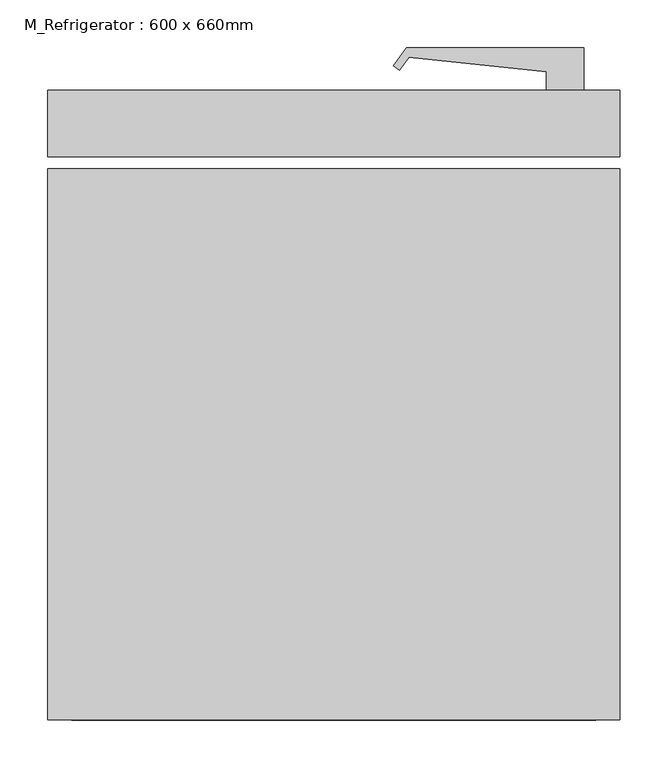
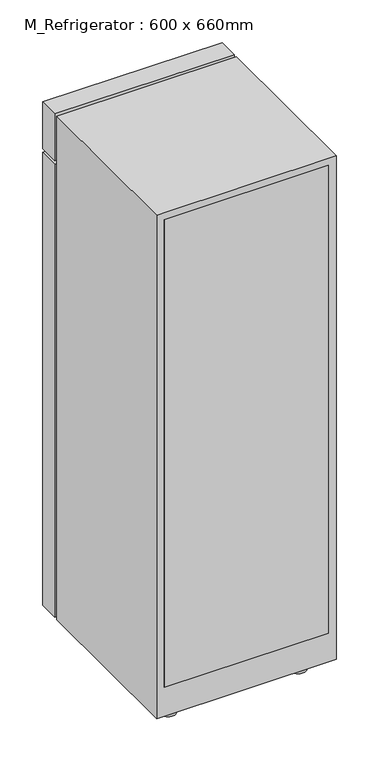
"""IFC4 building model written with IfcOpenShell, lengths in millimetres: proxy geometry, M_Refrigerator : 600 x 660mm."""

from ifc_helpers import new_model, si_unit, point, frame, frame_2d, origin, origin_with_axes, place, context, project, spatial, polyline, circle_curve, trimmed, segment, composite_curve, outline, extrude, source, transform, mapped, element, save


def m_refrigerator_600_x_660mm_0a899b9c(model_context):
    return source(origin(), model_context, "Body", "SweptSolid", [
        extrude(outline(polyline([(208.0988574, 408.1036861), (208.0988574, 363.7849098), (168.9242419, 363.7849098), (168.9242419, 383.0358618), (25.1756383, 398.2543926), (15.2273026, 384.7471068), (8.7240737, 389.5368406), (22.3988574, 408.1036861), (208.0988574, 408.1036861)])), frame((0.0, 0.0, 1071.927792), z_axis=(0.0, 0.0, 1.0), x_axis=(1.0, 0.0, 0.0)), (0.0, 0.0, 1.0), 31.75),
        extrude(outline(composite_curve([segment(trimmed(circle_curve(frame_2d((-271.2511426, -220.0150902)), 25.4), [point((-296.6511426, -220.0150902))], [point((-245.8511426, -220.0150902))], False, "CARTESIAN"), True, "CONTINUOUS"), segment(trimmed(circle_curve(frame_2d((-271.2511426, -220.0150902)), 25.4), [point((-245.8511426, -220.0150902))], [point((-296.6511426, -220.0150902))], False, "CARTESIAN"), True, "CONTINUOUS")], self_intersect=False)), origin_with_axes(), (0.0, 0.0, 1.0), 50.8),
        extrude(outline(composite_curve([segment(trimmed(circle_curve(frame_2d((163.6488574, -220.0150902)), 25.4), [point((138.2488574, -220.0150902))], [point((189.0488574, -220.0150902))], False, "CARTESIAN"), True, "CONTINUOUS"), segment(trimmed(circle_curve(frame_2d((163.6488574, -220.0150902)), 25.4), [point((189.0488574, -220.0150902))], [point((138.2488574, -220.0150902))], False, "CARTESIAN"), True, "CONTINUOUS")], self_intersect=False)), origin_with_axes(), (0.0, 0.0, 1.0), 50.8),
        extrude(outline(composite_curve([segment(trimmed(circle_curve(frame_2d((-271.2511426, 236.7849098)), 25.4), [point((-296.6511426, 236.7849098))], [point((-245.8511426, 236.7849098))], False, "CARTESIAN"), True, "CONTINUOUS"), segment(trimmed(circle_curve(frame_2d((-271.2511426, 236.7849098)), 25.4), [point((-245.8511426, 236.7849098))], [point((-296.6511426, 236.7849098))], False, "CARTESIAN"), True, "CONTINUOUS")], self_intersect=False)), origin_with_axes(), (0.0, 0.0, 1.0), 50.8),
        extrude(outline(composite_curve([segment(trimmed(circle_curve(frame_2d((163.6488574, 236.7849098)), 25.4), [point((138.2488574, 236.7849098))], [point((189.0488574, 236.7849098))], False, "CARTESIAN"), True, "CONTINUOUS"), segment(trimmed(circle_curve(frame_2d((163.6488574, 236.7849098)), 25.4), [point((189.0488574, 236.7849098))], [point((138.2488574, 236.7849098))], False, "CARTESIAN"), True, "CONTINUOUS")], self_intersect=False)), origin_with_axes(), (0.0, 0.0, 1.0), 50.8),
        extrude(outline(polyline([(246.1988574, 363.7849098), (246.1988574, 293.9349098), (-353.8011426, 293.9349098), (-353.8011426, 363.7849098), (246.1988574, 363.7849098)])), frame((0.0, 0.0, 50.8), z_axis=(0.0, 0.0, 1.0), x_axis=(1.0, 0.0, 0.0)), (0.0, 0.0, 1.0), 1601.4),
        extrude(outline(polyline([(246.1988574, 363.7849098), (246.1988574, 293.9349098), (-353.8011426, 293.9349098), (-353.8011426, 363.7849098), (246.1988574, 363.7849098)])), frame((0.0, 0.0, 1664.9), z_axis=(0.0, 0.0, 1.0), x_axis=(1.0, 0.0, 0.0)), (0.0, 0.0, 1.0), 165.1),
        extrude(outline(polyline([(220.7988574, -270.8150902), (220.7988574, -296.2150902), (-328.4011426, -296.2150902), (-328.4011426, -270.8150902), (220.7988574, -270.8150902)])), frame((0.0, 0.0, 152.4), z_axis=(0.0, 0.0, 1.0), x_axis=(1.0, 0.0, 0.0)), (0.0, 0.0, 1.0), 1652.2),
        extrude(outline(polyline([(1830.0, 246.1988574), (1830.0, -353.8011426), (50.8, -353.8011426), (50.8, 246.1988574), (1830.0, 246.1988574)]), holes=[polyline([(1626.8, 220.7988574), (431.8, 220.7988574), (431.8, -328.4011426), (1626.8, -328.4011426), (1626.8, 220.7988574)])]), frame((0.0, -296.2150902, 0.0), z_axis=(0.0, 1.0, 0.0), x_axis=(0.0, 0.0, 1.0)), (0.0, 0.0, 1.0), 577.45),
    ])


if __name__ == "__main__":
    model = new_model("IFC4")
    model_context = context("Model", 3, world=origin())
    ifc_project = project(units=[si_unit("LENGTHUNIT", "METRE", prefix="MILLI")], contexts=[model_context])
    site = spatial("IfcSite", under=ifc_project)
    building = spatial("IfcBuilding", under=site)
    placement = place(None, origin())
    m_refrigerator_600_x_660mm_shape = m_refrigerator_600_x_660mm_0a899b9c(model_context)
    element("IfcBuildingElementProxy", 1, Name="M_Refrigerator : 600 x 660mm", ObjectType="M_Refrigerator : 600 x 660mm", at=placement, inside=building, context=model_context, shape_type="MappedRepresentation", body=[
        mapped(m_refrigerator_600_x_660mm_shape, transform((0.0, 0.0, 0.0), x_axis=(1.0, 0.0, 0.0), y_axis=(0.0, 1.0, 0.0), z_axis=(0.0, 0.0, 1.0))),
    ])
    save(model, "model.ifc")

# Revit data of these elements
# Type "M_Refrigerator : 600 x 660mm"
#   Label = "REF."
#   Depth = 2.165354 ft
#   Height = 6.003937 ft
#   Width = 1.968504 ft
#   Material = Steel, Paint Finish, Ivory, Matte
#   Description = (empty or 0)
#   Default Elevation = 0
# Element 1 (IfcBuildingElementProxy, "M_Refrigerator : 600 x 660mm")
#   Materials on its faces: "Steel, Paint Finish, Ivory, Matte", "Steel, Chrome Plated"
# Materials
#   "Steel, Paint Finish, Ivory, Matte": class "Metal", colour RGB 247 247 239, transparency 0, Description = "Steel, paint finish, ivory, matte", Cost = 0
#   "Steel, Chrome Plated": class "Metal", colour RGB 17 17 17, transparency 0, Description = "Chromiuim plated steel", Cost = 0
